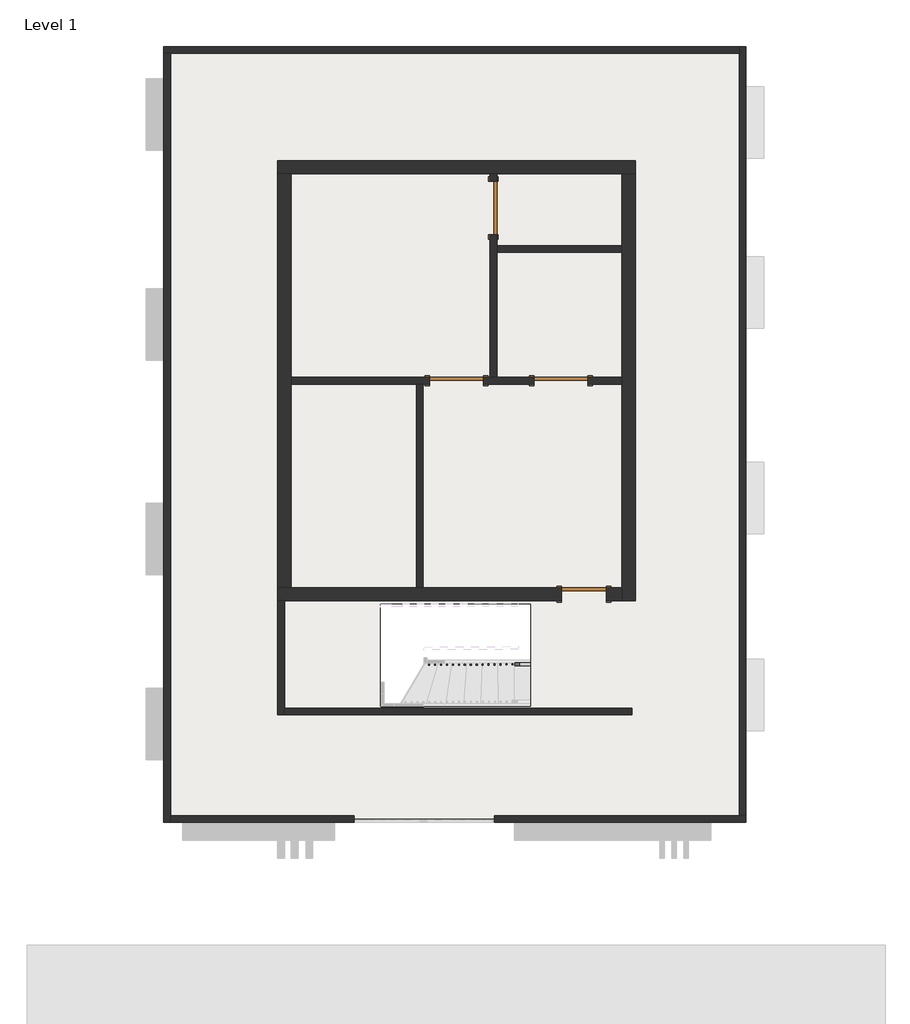
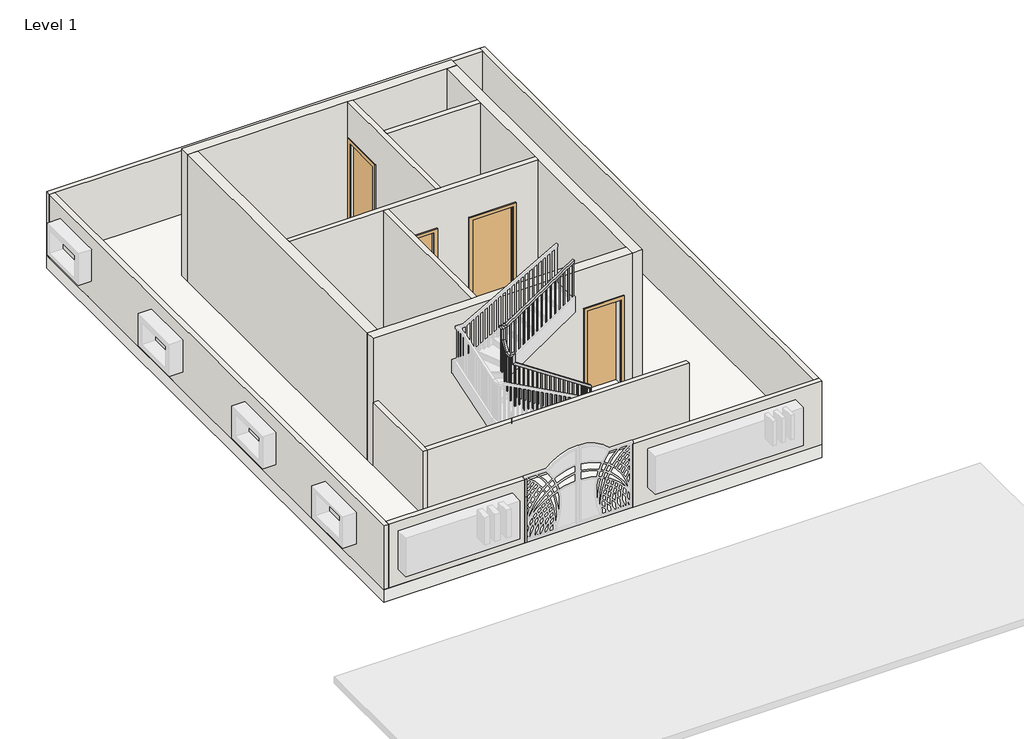
# One storey, part 1 of 2: 15 walls, 4 doors, 1 railing, 1 slab.
"""IFC4 building model written with IfcOpenShell, lengths in millimetres."""

from ifc_helpers import new_model, si_unit, frame, origin, origin_with_axes, place, context, project, spatial, polyline, outline, extrude, faceted_brep, transform, mapped, element, save
from components import door_a1484949, door_e5f9f3c4, door_305aa2a5

model = new_model("IFC4")

# Units and contexts
model_context = context("Model", 3, world=origin())
ifc_project = project(units=[si_unit("LENGTHUNIT", "METRE", prefix="MILLI")], contexts=[model_context])

# Site, building, storey
site = spatial("IfcSite", under=ifc_project)
building = spatial("IfcBuilding", under=site)
storey = spatial("IfcBuildingStorey", under=building, Name="Level 1", Elevation=0.0)

# Doors
placement = place(None, origin())
door_shape = door_a1484949(model_context)
element("IfcDoor", 1, ObjectType="Single-Flush : 30\" x 80\"", at=placement, inside=storey, context=model_context, shape_type="MappedRepresentation", body=[
    mapped(door_shape, transform((792.5410386, -2372.0109248, 0.0), x_axis=(1.0, 0.0, 0.0), y_axis=(0.0, 1.0, 0.0), z_axis=(0.0, 0.0, 1.0))),
])
door_2_shape = door_e5f9f3c4(model_context)
element("IfcDoor", 2, ObjectType="Single-Flush : 36\" x 84\"", at=placement, inside=storey, context=model_context, shape_type="MappedRepresentation", body=[
    mapped(door_2_shape, transform((-750.5089614, 4209.7640752, 0.0), x_axis=(0.0, -1.0, 0.0), y_axis=(1.0, 0.0, 0.0), z_axis=(0.0, 0.0, 1.0))),
])
door_3_shape = door_305aa2a5(model_context)
element("IfcDoor", 3, ObjectType="Single-Flush : 36\" x 84\"", at=placement, inside=storey, context=model_context, shape_type="MappedRepresentation", body=[
    mapped(door_3_shape, transform((402.0160386, 1266.5390752, 0.0), x_axis=(-1.0, 0.0, 0.0), y_axis=(0.0, -1.0, 0.0), z_axis=(0.0, 0.0, 1.0))),
])
element("IfcDoor", 4, ObjectType="Single-Flush : 36\" x 84\"", at=placement, inside=storey, context=model_context, shape_type="MappedRepresentation", body=[
    mapped(door_3_shape, transform((-1379.1589614, 1266.5390752, 0.0), x_axis=(-1.0, 0.0, 0.0), y_axis=(0.0, -1.0, 0.0), z_axis=(0.0, 0.0, 1.0))),
])

# Railing
element("IfcRailing", 5, ObjectType="Handrail - Rectangular", at=placement, inside=storey, context=model_context, shape_type="SolidModel", body=[
    faceted_brep([(-120.3816305, -3590.4209536, 1083.7333333), (-120.3816305, -3590.4209536, 1022.5630107), (-120.6930289, -3539.621908, 1022.5630107), (-120.6930289, -3539.621908, 1083.7333333), (-1854.5612186, -3601.0514854, 2247.0182998), (-1905.3602642, -3601.3628839, 2219.9238978), (-1905.6716627, -3550.5638383, 2219.9238978), (-1854.8726171, -3550.2524399, 2247.0182998), (-1854.5612186, -3601.0514854, 2469.2829276), (-1905.3602642, -3601.3628839, 2418.4829276), (-1905.6716627, -3550.5638383, 2418.4829276), (-1854.8726171, -3550.2524399, 2469.2829276), (-1981.5588325, -3601.8299816, 2469.2829276), (-1981.5588325, -3601.8299816, 2418.4829276), (-1931.0711854, -3550.7195376, 2418.4829276), (-1931.0711854, -3550.7195376, 2469.2829276), (-1982.3373287, -3474.8323677, 2469.2829276), (-1982.5128182, -3446.2044317, 2418.4829276), (-1931.7137726, -3445.8930332, 2418.4829276), (-1931.5382832, -3474.5209692, 2469.2829276), (-1983.1158249, -3347.8347538, 2679.0434812), (-1983.4272234, -3297.0357082, 2664.8632575), (-1932.6281778, -3296.7243097, 2664.8632575), (-1932.3167793, -3347.5233553, 2679.0434812), (-1983.1158249, -3347.8347538, 2950.4951436), (-1983.4272234, -3297.0357082, 2899.6951436), (-1932.6281778, -3296.7243097, 2899.6951436), (-1932.3167793, -3347.5233553, 2950.4951436), (-1983.8943211, -3220.8371398, 2950.4951436), (-1983.8943211, -3220.8371398, 2899.6951436), (-1932.783877, -3271.3247869, 2899.6951436), (-1932.783877, -3271.3247869, 2950.4951436), (-1856.8967072, -3220.0586437, 2950.4951436), (-1841.6341703, -3219.9650842, 2899.6951436), (-1841.3227719, -3270.7641298, 2899.6951436), (-1856.5853087, -3270.8576892, 2950.4951436), (-324.9523945, -3210.6678153, 3962.4), (-324.6409961, -3261.4668609, 3962.4), (-324.6409961, -3261.4668609, 3901.5185401), (-324.9523945, -3210.6678153, 3901.5185401)], [[[0, 1, 2, 3]], [[1, 0, 4, 5]], [[2, 1, 5, 6]], [[3, 2, 6, 7]], [[0, 3, 7, 4]], [[5, 4, 8, 9]], [[6, 5, 9, 10]], [[7, 6, 10, 11]], [[4, 7, 11, 8]], [[9, 8, 12, 13]], [[10, 9, 13, 14]], [[11, 10, 14, 15]], [[8, 11, 15, 12]], [[13, 12, 16, 17]], [[14, 13, 17, 18]], [[15, 14, 18, 19]], [[12, 15, 19, 16]], [[17, 16, 20, 21]], [[18, 17, 21, 22]], [[19, 18, 22, 23]], [[16, 19, 23, 20]], [[21, 20, 24, 25]], [[22, 21, 25, 26]], [[23, 22, 26, 27]], [[20, 23, 27, 24]], [[25, 24, 28, 29]], [[26, 25, 29, 30]], [[27, 26, 30, 31]], [[24, 27, 31, 28]], [[29, 28, 32, 33]], [[30, 29, 33, 34]], [[31, 30, 34, 35]], [[28, 31, 35, 32]], [[36, 37, 38, 39]], [[33, 32, 36, 39]], [[34, 33, 39, 38]], [[35, 34, 38, 37]], [[32, 35, 37, 36]]]),
    extrude(outline(polyline([(222.3085098, -19.05), (234.8914903, 0.0), (1246.1854534, 0.0), (1246.1854534, -19.05), (222.3085098, -19.05)])), frame((-342.2360746, -3245.6994205, 4124.8521201), z_axis=(-0.00612989118043648, 0.9999812120405643, 0.0), x_axis=(0.0, 0.0, -1.0)), (0.0, 0.0, 1.0), 19.05),
    extrude(outline(polyline([(222.3085098, -19.0499999), (234.8914902, 0.0), (1179.0762243, 0.0), (1179.0762243, -19.0499999), (222.3085098, -19.0499999)])), frame((-443.8341657, -3246.3222175, 4057.742891), z_axis=(-0.00612989118043648, 0.9999812120405643, 0.0), x_axis=(0.0, 0.0, -1.0)), (0.0, 0.0, 1.0), 19.05),
    extrude(outline(polyline([(222.3085098, -19.05), (234.8914902, 0.0), (1111.9669952, 0.0), (1111.9669952, -19.05), (222.3085098, -19.05)])), frame((-545.4322569, -3246.9450144, 3990.6336619), z_axis=(-0.00612989118043648, 0.9999812120405643, 0.0), x_axis=(0.0, 0.0, -1.0)), (0.0, 0.0, 1.0), 19.05),
    extrude(outline(polyline([(222.3085098, -19.05), (234.8914902, 0.0), (1214.1910995, 0.0), (1214.1910995, -19.05), (222.3085098, -19.05)])), frame((-647.030348, -3247.5678114, 3923.5244328), z_axis=(-0.00612989118043648, 0.9999812120405643, 0.0), x_axis=(0.0, 0.0, -1.0)), (0.0, 0.0, 1.0), 19.05),
    extrude(outline(polyline([(222.3085098, -19.05), (234.8914902, 0.0), (1147.0818704, 0.0), (1147.0818704, -19.05), (222.3085098, -19.05)])), frame((-748.6284392, -3248.1906083, 3856.4152037), z_axis=(-0.00612989118043648, 0.9999812120405643, 0.0), x_axis=(0.0, 0.0, -1.0)), (0.0, 0.0, 1.0), 19.05),
    extrude(outline(polyline([(222.3085098, -19.05), (234.8914902, 0.0), (1079.9726413, 0.0), (1079.9726413, -19.05), (222.3085098, -19.05)])), frame((-850.2265303, -3248.8134053, 3789.3059746), z_axis=(-0.00612989118043648, 0.9999812120405643, 0.0), x_axis=(0.0, 0.0, -1.0)), (0.0, 0.0, 1.0), 19.05),
    extrude(outline(polyline([(222.3085098, -19.05), (234.8914902, 0.0), (1182.1967455, 0.0), (1182.1967455, -19.05), (222.3085098, -19.05)])), frame((-951.8246215, -3249.4362022, 3722.1967455), z_axis=(-0.00612989118043648, 0.9999812120405643, 0.0), x_axis=(0.0, 0.0, -1.0)), (0.0, 0.0, 1.0), 19.05),
    extrude(outline(polyline([(222.3085097, -19.05), (234.8914902, 0.0), (1115.0875164, 0.0), (1115.0875164, -19.05), (222.3085097, -19.05)])), frame((-1053.4227126, -3250.0589992, 3655.0875164), z_axis=(-0.00612989118043648, 0.9999812120405643, 0.0), x_axis=(0.0, 0.0, -1.0)), (0.0, 0.0, 1.0), 19.05),
    extrude(outline(polyline([(222.3085097, -19.0499999), (234.8914902, 0.0), (1047.9782873, 0.0), (1047.9782873, -19.0499999), (222.3085097, -19.0499999)])), frame((-1155.0208037, -3250.6817961, 3587.9782873), z_axis=(-0.00612989118043648, 0.9999812120405643, 0.0), x_axis=(0.0, 0.0, -1.0)), (0.0, 0.0, 1.0), 19.05),
    extrude(outline(polyline([(222.3085097, -19.05), (234.8914902, 0.0), (1150.2023915, 0.0), (1150.2023915, -19.05), (222.3085097, -19.05)])), frame((-1256.6188949, -3251.304593, 3520.8690582), z_axis=(-0.00612989118043648, 0.9999812120405643, 0.0), x_axis=(0.0, 0.0, -1.0)), (0.0, 0.0, 1.0), 19.05),
    extrude(outline(polyline([(222.3085098, -19.05), (234.8914903, 0.0), (1083.0931625, 0.0), (1083.0931625, -19.05), (222.3085098, -19.05)])), frame((-1358.216986, -3251.92739, 3453.7598292), z_axis=(-0.00612989118043648, 0.9999812120405643, 0.0), x_axis=(0.0, 0.0, -1.0)), (0.0, 0.0, 1.0), 19.05),
    extrude(outline(polyline([(222.3085098, -19.05), (234.8914903, 0.0), (1185.3172668, 0.0), (1185.3172668, -19.05), (222.3085098, -19.05)])), frame((-1459.8150772, -3252.5501869, 3386.6506001), z_axis=(-0.00612989118043648, 0.9999812120405643, 0.0), x_axis=(0.0, 0.0, -1.0)), (0.0, 0.0, 1.0), 19.05),
    extrude(outline(polyline([(222.3085098, -19.05), (234.8914903, 0.0), (1118.2080377, 0.0), (1118.2080377, -19.05), (222.3085098, -19.05)])), frame((-1561.4131683, -3253.1729839, 3319.541371), z_axis=(-0.00612989118043648, 0.9999812120405643, 0.0), x_axis=(0.0, 0.0, -1.0)), (0.0, 0.0, 1.0), 19.05),
    extrude(outline(polyline([(222.3085098, -19.05), (234.8914902, 0.0), (1051.0988086, 0.0), (1051.0988086, -19.05), (222.3085098, -19.05)])), frame((-1663.0112595, -3253.7957808, 3252.4321419), z_axis=(-0.00612989118043648, 0.9999812120405643, 0.0), x_axis=(0.0, 0.0, -1.0)), (0.0, 0.0, 1.0), 19.05),
    extrude(outline(polyline([(222.3085098, -19.05), (234.8914902, 0.0), (1153.3229128, 0.0), (1153.3229128, -19.05), (222.3085098, -19.05)])), frame((-1764.6093506, -3254.4185778, 3185.3229128), z_axis=(-0.00612989118043648, 0.9999812120405643, 0.0), x_axis=(0.0, 0.0, -1.0)), (0.0, 0.0, 1.0), 19.05),
    extrude(outline(polyline([(222.3085098, -19.05), (234.8914902, 0.0), (1086.2136837, 0.0), (1086.2136837, -19.05), (222.3085098, -19.05)])), frame((-1866.2074418, -3255.0413747, 3118.2136837), z_axis=(-0.00612989118043648, 0.9999812120405643, 0.0), x_axis=(0.0, 0.0, -1.0)), (0.0, 0.0, 1.0), 19.05),
    extrude(outline(polyline([(-1948.6001916, -3280.94692), (-1967.6498337, -3281.0636944), (-1967.7666081, -3262.0140523), (-1948.716966, -3261.8972779), (-1948.6001916, -3280.94692)])), frame((0.0, 0.0, 1862.6666667), z_axis=(0.0, 0.0, 1.0), x_axis=(1.0, 0.0, 0.0)), (0.0, 0.0, 1.0), 1037.0284769),
    extrude(outline(polyline([(244.3320415, -19.05), (212.8679585, 0.0), (1074.2735921, 0.0), (1074.2735921, -19.05), (244.3320415, -19.05)])), frame((-1967.1438111, -3363.6121435, 2767.6069254), z_axis=(0.9999812120405644, 0.006129891180436036, 0.0), x_axis=(0.0, 0.0, -1.0)), (0.0, 0.0, 1.0), 19.05),
    extrude(outline(polyline([(244.3320415, -19.05), (212.8679585, 0.0), (1075.7984825, 0.0), (1075.7984825, -19.05), (244.3320415, -19.05)])), frame((-1966.5210142, -3465.2102346, 2599.7984825), z_axis=(0.9999812120405644, 0.006129891180436036, 0.0), x_axis=(0.0, 0.0, -1.0)), (0.0, 0.0, 1.0), 19.05),
    extrude(outline(polyline([(-1939.8365364, -3566.6485675), (-1939.719762, -3585.6982096), (-1958.7694041, -3585.814984), (-1958.8861785, -3566.7653419), (-1939.8365364, -3566.6485675)])), frame((0.0, 0.0, 1354.6666667), z_axis=(0.0, 0.0, 1.0), x_axis=(1.0, 0.0, 0.0)), (0.0, 0.0, 1.0), 1063.816261),
    extrude(outline(polyline([(234.9892351, -19.05), (222.2107648, 0.0), (1224.4109792, 0.0), (1224.4109792, -19.05), (234.9892351, -19.05)])), frame((-1857.171313, -3585.1921871, 2409.7443125), z_axis=(-0.006129891180436334, 0.9999812120405643, 0.0), x_axis=(0.0, 0.0, -1.0)), (0.0, 0.0, 1.0), 19.05),
    extrude(outline(polyline([(234.9892352, -19.05), (222.2107649, 0.0), (1156.259138, 0.0), (1156.259138, -19.05), (234.9892352, -19.05)])), frame((-1755.5732218, -3584.5693901, 2341.5924713), z_axis=(-0.006129891180436334, 0.9999812120405643, 0.0), x_axis=(0.0, 0.0, -1.0)), (0.0, 0.0, 1.0), 19.05),
    extrude(outline(polyline([(234.9892351, -19.05), (222.2107649, 0.0), (1257.44063, 0.0), (1257.44063, -19.05), (234.9892351, -19.05)])), frame((-1653.9751307, -3583.9465932, 2273.44063), z_axis=(-0.006129891180436334, 0.9999812120405643, 0.0), x_axis=(0.0, 0.0, -1.0)), (0.0, 0.0, 1.0), 19.05),
    extrude(outline(polyline([(234.9892351, -19.05), (222.2107649, 0.0), (1189.2887887, 0.0), (1189.2887887, -19.05), (234.9892351, -19.05)])), frame((-1552.3770395, -3583.3237962, 2205.2887887), z_axis=(-0.006129891180436334, 0.9999812120405643, 0.0), x_axis=(0.0, 0.0, -1.0)), (0.0, 0.0, 1.0), 19.05),
    extrude(outline(polyline([(234.9892351, -19.05), (222.2107649, 0.0), (1290.4702807, 0.0), (1290.4702807, -19.05), (234.9892351, -19.05)])), frame((-1450.7789484, -3582.7009993, 2137.1369474), z_axis=(-0.006129891180436334, 0.9999812120405643, 0.0), x_axis=(0.0, 0.0, -1.0)), (0.0, 0.0, 1.0), 19.05),
    extrude(outline(polyline([(234.9892351, -19.0499999), (222.2107649, 0.0), (1222.3184394, 0.0), (1222.3184394, -19.0499999), (234.9892351, -19.0499999)])), frame((-1349.1808572, -3582.0782024, 2068.9851061), z_axis=(-0.006129891180436334, 0.9999812120405643, 0.0), x_axis=(0.0, 0.0, -1.0)), (0.0, 0.0, 1.0), 19.05),
    extrude(outline(polyline([(234.9892351, -19.05), (222.2107648, 0.0), (1154.1665981, 0.0), (1154.1665981, -19.05), (234.9892351, -19.05)])), frame((-1247.5827661, -3581.4554054, 2000.8332648), z_axis=(-0.006129891180436334, 0.9999812120405643, 0.0), x_axis=(0.0, 0.0, -1.0)), (0.0, 0.0, 1.0), 19.05),
    extrude(outline(polyline([(234.9892352, -19.05), (222.2107649, 0.0), (1255.3480903, 0.0), (1255.3480903, -19.05), (234.9892352, -19.05)])), frame((-1145.984675, -3580.8326085, 1932.6814236), z_axis=(-0.006129891180436334, 0.9999812120405643, 0.0), x_axis=(0.0, 0.0, -1.0)), (0.0, 0.0, 1.0), 19.05),
    extrude(outline(polyline([(234.9892351, -19.05), (222.2107649, 0.0), (1187.196249, 0.0), (1187.196249, -19.05), (234.9892351, -19.05)])), frame((-1044.3865838, -3580.2098115, 1864.5295823), z_axis=(-0.006129891180436334, 0.9999812120405643, 0.0), x_axis=(0.0, 0.0, -1.0)), (0.0, 0.0, 1.0), 19.05),
    extrude(outline(polyline([(234.9892351, -19.05), (222.2107649, 0.0), (1288.377741, 0.0), (1288.377741, -19.05), (234.9892351, -19.05)])), frame((-942.7884927, -3579.5870146, 1796.377741), z_axis=(-0.006129891180436334, 0.9999812120405643, 0.0), x_axis=(0.0, 0.0, -1.0)), (0.0, 0.0, 1.0), 19.05),
    extrude(outline(polyline([(234.9892351, -19.05), (222.2107649, 0.0), (1220.2258997, 0.0), (1220.2258997, -19.05), (234.9892351, -19.05)])), frame((-841.1904015, -3578.9642176, 1728.2258997), z_axis=(-0.006129891180436334, 0.9999812120405643, 0.0), x_axis=(0.0, 0.0, -1.0)), (0.0, 0.0, 1.0), 19.05),
    extrude(outline(polyline([(234.9892351, -19.05), (222.2107649, 0.0), (1152.0740584, 0.0), (1152.0740584, -19.05), (234.9892351, -19.05)])), frame((-739.5923104, -3578.3414207, 1660.0740584), z_axis=(-0.006129891180436334, 0.9999812120405643, 0.0), x_axis=(0.0, 0.0, -1.0)), (0.0, 0.0, 1.0), 19.05),
    extrude(outline(polyline([(234.9892351, -19.0499999), (222.2107648, 0.0), (1253.2555504, 0.0), (1253.2555504, -19.0499999), (234.9892351, -19.0499999)])), frame((-637.9942192, -3577.7186237, 1591.9222171), z_axis=(-0.006129891180436334, 0.9999812120405643, 0.0), x_axis=(0.0, 0.0, -1.0)), (0.0, 0.0, 1.0), 19.05),
    extrude(outline(polyline([(234.9892352, -19.05), (222.2107649, 0.0), (1185.1037092, 0.0), (1185.1037092, -19.05), (234.9892352, -19.05)])), frame((-536.3961281, -3577.0958268, 1523.7703759), z_axis=(-0.006129891180436334, 0.9999812120405643, 0.0), x_axis=(0.0, 0.0, -1.0)), (0.0, 0.0, 1.0), 19.05),
    extrude(outline(polyline([(234.9892351, -19.05), (222.2107649, 0.0), (1116.9518679, 0.0), (1116.9518679, -19.05), (234.9892351, -19.05)])), frame((-434.798037, -3576.4730299, 1455.6185346), z_axis=(-0.006129891180436334, 0.9999812120405643, 0.0), x_axis=(0.0, 0.0, -1.0)), (0.0, 0.0, 1.0), 19.05),
    extrude(outline(polyline([(234.9892351, -19.05), (222.2107649, 0.0), (1218.13336, 0.0), (1218.13336, -19.05), (234.9892351, -19.05)])), frame((-333.1999458, -3575.8502329, 1387.4666933), z_axis=(-0.006129891180436334, 0.9999812120405643, 0.0), x_axis=(0.0, 0.0, -1.0)), (0.0, 0.0, 1.0), 19.05),
    extrude(outline(polyline([(234.9892351, -19.05), (222.2107649, 0.0), (1149.9815187, 0.0), (1149.9815187, -19.05), (234.9892351, -19.05)])), frame((-231.6018547, -3575.227436, 1319.314852), z_axis=(-0.006129891180436334, 0.9999812120405643, 0.0), x_axis=(0.0, 0.0, -1.0)), (0.0, 0.0, 1.0), 19.05),
    extrude(outline(polyline([(-1948.7558908, -3255.5473972), (-1967.8055329, -3255.6641716), (-1967.9223073, -3236.6145296), (-1948.8726652, -3236.4977551), (-1948.7558908, -3255.5473972)])), frame((0.0, 0.0, 1862.6666667), z_axis=(0.0, 0.0, 1.0), x_axis=(1.0, 0.0, 0.0)), (0.0, 0.0, 1.0), 1037.0284769),
    extrude(outline(polyline([(-1946.8485752, -3566.6915513), (-1946.7318007, -3585.7411934), (-1965.7814428, -3585.8579679), (-1965.8982173, -3566.8083258), (-1946.8485752, -3566.6915513)])), frame((0.0, 0.0, 1354.6666667), z_axis=(0.0, 0.0, 1.0), x_axis=(1.0, 0.0, 0.0)), (0.0, 0.0, 1.0), 1063.816261),
    extrude(outline(polyline([(222.3085098, -19.05), (234.8914902, 0.0), (1245.1603832, 0.0), (1245.1603832, -19.05), (222.3085098, -19.05)])), frame((-343.7879502, -3245.7089335, 4123.8270499), z_axis=(-0.00612989118043648, 0.9999812120405643, 0.0), x_axis=(0.0, 0.0, -1.0)), (0.0, 0.0, 1.0), 19.05),
    extrude(outline(polyline([(234.9892351, -19.05), (222.2107648, 0.0), (1088.2189125, 0.0), (1088.2189125, -19.05), (234.9892351, -19.05)])), frame((-139.5285846, -3574.6630262, 1257.5522458), z_axis=(-0.006129891180436334, 0.9999812120405643, 0.0), x_axis=(0.0, 0.0, -1.0)), (0.0, 0.0, 1.0), 19.05),
])

# Slab
element("IfcSlab", 6, ObjectType="Generic - 12\"", at=placement, inside=storey, context=model_context, shape_type="SweptSolid", body=[
    extrude(outline(polyline([(3554.7910386, 6962.4890752), (3554.7910386, -6258.2109248), (-6370.2589614, -6258.2109248), (-6370.2589614, 6962.4890752), (3554.7910386, 6962.4890752)]), holes=[polyline([(-116.1777511, -2539.253904), (-2673.8853157, -2539.253904), (-2673.8853157, -4276.2080688), (-116.1777511, -4276.2080688), (-116.1777511, -2539.253904)])]), frame((0.0, 0.0, -304.8), z_axis=(0.0, 0.0, 1.0), x_axis=(1.0, 0.0, 0.0)), (0.0, 0.0, 1.0), 304.8),
])

# Walls
element("IfcWall", 7, ObjectType="4.5\"", at=placement, inside=storey, context=model_context, shape_type="Brep", body=[
    faceted_brep([(-807.6589614, 3752.5640752, 2133.6), (-807.6589614, 3752.5640752, 0.0), (-807.6589614, 1323.6890752, 0.0), (-807.6589614, 1323.6890752, 3048.0), (-807.6589614, 4790.7890752, 3048.0), (-807.6589614, 4790.7890752, 0.0), (-807.6589614, 4666.9640752, 0.0), (-807.6589614, 4666.9640752, 2133.6), (-693.3589614, 1323.6890752, 0.0), (-693.3589614, 3457.2890752, 0.0), (-693.3589614, 3571.5890752, 0.0), (-693.3589614, 3752.5640752, 0.0), (-693.3589614, 3752.5640752, 2133.6), (-693.3589614, 4666.9640752, 2133.6), (-693.3589614, 4666.9640752, 0.0), (-693.3589614, 4790.7890752, 0.0), (-693.3589614, 4790.7890752, 3048.0), (-693.3589614, 3571.5890752, 3048.0), (-693.3589614, 3457.2890752, 3048.0), (-693.3589614, 1323.6890752, 3048.0)], [[[0, 1, 2, 3, 4, 5, 6, 7]], [[8, 9, 10, 11, 12, 13, 14, 15, 16, 17, 18, 19]], [[6, 5, 15, 14]], [[2, 1, 11, 10, 9, 8]], [[5, 4, 16, 15]], [[3, 2, 8, 19]], [[12, 11, 1, 0]], [[13, 12, 0, 7]], [[14, 13, 7, 6]], [[4, 3, 19, 18, 17, 16]]]),
])
element("IfcWall", 8, ObjectType="4.5\"", at=placement, inside=storey, context=model_context, shape_type="SweptSolid", body=[
    extrude(outline(polyline([(-693.3589614, 3571.5890752), (1440.2410386, 3571.5890752), (1440.2410386, 3457.2890752), (-693.3589614, 3457.2890752), (-693.3589614, 3571.5890752)])), origin_with_axes(), (0.0, 0.0, 1.0), 3048.0),
])
element("IfcWall", 9, ObjectType="4.5\"", at=placement, inside=storey, context=model_context, shape_type="Brep", body=[
    faceted_brep([(-4198.5589614, 1209.3890752, 0.0), (-2064.9589614, 1209.3890752, 0.0), (-1950.6589614, 1209.3890752, 0.0), (-1836.3589614, 1209.3890752, 0.0), (-1836.3589614, 1209.3890752, 2133.6), (-921.9589614, 1209.3890752, 2133.6), (-921.9589614, 1209.3890752, 0.0), (-55.1839614, 1209.3890752, 0.0), (-55.1839614, 1209.3890752, 2133.6), (859.2160386, 1209.3890752, 2133.6), (859.2160386, 1209.3890752, 0.0), (1440.2410386, 1209.3890752, 0.0), (1440.2410386, 1209.3890752, 3048.0), (-1950.6589614, 1209.3890752, 3048.0), (-2064.9589614, 1209.3890752, 3048.0), (-4198.5589614, 1209.3890752, 3048.0), (-1836.3589614, 1323.6890752, 2133.6), (-1836.3589614, 1323.6890752, 0.0), (-4198.5589614, 1323.6890752, 0.0), (-4198.5589614, 1323.6890752, 3048.0), (-807.6589614, 1323.6890752, 3048.0), (-693.3589614, 1323.6890752, 3048.0), (1440.2410386, 1323.6890752, 3048.0), (1440.2410386, 1323.6890752, 0.0), (859.2160386, 1323.6890752, 0.0), (859.2160386, 1323.6890752, 2133.6), (-55.1839614, 1323.6890752, 2133.6), (-55.1839614, 1323.6890752, 0.0), (-693.3589614, 1323.6890752, 0.0), (-807.6589614, 1323.6890752, 0.0), (-921.9589614, 1323.6890752, 0.0), (-921.9589614, 1323.6890752, 2133.6)], [[[0, 1, 2, 3, 4, 5, 6, 7, 8, 9, 10, 11, 12, 13, 14, 15]], [[16, 17, 18, 19, 20, 21, 22, 23, 24, 25, 26, 27, 28, 29, 30, 31]], [[24, 23, 11, 10]], [[18, 17, 3, 2, 1, 0]], [[30, 29, 28, 27, 7, 6]], [[12, 11, 23, 22]], [[0, 15, 19, 18]], [[8, 7, 27, 26]], [[9, 8, 26, 25]], [[10, 9, 25, 24]], [[4, 3, 17, 16]], [[5, 4, 16, 31]], [[6, 5, 31, 30]], [[15, 14, 13, 12, 22, 21, 20, 19]]]),
])
element("IfcWall", 10, ObjectType="4.5\"", at=placement, inside=storey, context=model_context, shape_type="SweptSolid", body=[
    extrude(outline(polyline([(-2064.9589614, -2257.7109248), (-2064.9589614, 1209.3890752), (-1950.6589614, 1209.3890752), (-1950.6589614, -2257.7109248), (-2064.9589614, -2257.7109248)])), origin_with_axes(), (0.0, 0.0, 1.0), 3048.0),
])
element("IfcWall", 11, ObjectType="4.5\"", at=placement, inside=storey, context=model_context, shape_type="Brep", body=[
    faceted_brep([(-4427.1589614, -2486.3109248, 0.0), (-4427.1589614, -4429.4109248, 0.0), (-4427.1589614, -4429.4109248, 1524.0), (-4427.1589614, -2486.3109248, 1524.0), (-4312.8589614, -2486.3109248, 0.0), (-4312.8589614, -2486.3109248, 1524.0), (-4312.8589614, -4315.1109248, 1524.0), (-4312.8589614, -4429.4109248, 1524.0), (-4312.8589614, -4429.4109248, 0.0), (-4312.8589614, -4315.1109248, 0.0)], [[[0, 1, 2, 3]], [[4, 5, 6, 7, 8, 9]], [[1, 0, 4, 9, 8]], [[3, 2, 7, 6, 5]], [[0, 3, 5, 4]], [[2, 1, 8, 7]]]),
])
element("IfcWall", 12, ObjectType="4.5\"", at=placement, inside=storey, context=model_context, shape_type="SweptSolid", body=[
    extrude(outline(polyline([(1611.6910386, -4429.4109248), (-4312.8589614, -4429.4109248), (-4312.8589614, -4315.1109248), (1611.6910386, -4315.1109248), (1611.6910386, -4429.4109248)])), origin_with_axes(), (0.0, 0.0, 1.0), 1524.0),
])
element("IfcWall", 13, ObjectType="4.5\"", at=placement, inside=storey, context=model_context, shape_type="Brep", body=[
    faceted_brep([(-6370.2589614, 6848.1890752, 0.0), (-6255.9589614, 6848.1890752, 0.0), (3440.4910386, 6848.1890752, 0.0), (3440.4910386, 6848.1890752, 1524.0), (-6255.9589614, 6848.1890752, 1524.0), (-6370.2589614, 6848.1890752, 1524.0), (-6370.2589614, 6962.4890752, 0.0), (-6370.2589614, 6962.4890752, 1524.0), (3440.4910386, 6962.4890752, 1524.0), (3440.4910386, 6962.4890752, 0.0)], [[[0, 1, 2, 3, 4, 5]], [[6, 7, 8, 9]], [[2, 1, 0, 6, 9]], [[5, 4, 3, 8, 7]], [[0, 5, 7, 6]], [[3, 2, 9, 8]]]),
])
element("IfcWall", 14, ObjectType="4.5\"", at=placement, inside=storey, context=model_context, shape_type="Brep", body=[
    faceted_brep([(-6255.9589614, -6258.2109248, 0.0), (-6255.9589614, -6143.9109248, 0.0), (-6255.9589614, 6848.1890752, 0.0), (-6255.9589614, 6848.1890752, 1524.0), (-6255.9589614, -6143.9109248, 1524.0), (-6255.9589614, -6258.2109248, 1524.0), (-6370.2589614, -6258.2109248, 0.0), (-6370.2589614, -6258.2109248, 1524.0), (-6370.2589614, 6848.1890752, 1524.0), (-6370.2589614, 6848.1890752, 0.0)], [[[0, 1, 2, 3, 4, 5]], [[6, 7, 8, 9]], [[2, 1, 0, 6, 9]], [[5, 4, 3, 8, 7]], [[0, 5, 7, 6]], [[3, 2, 9, 8]]]),
])
element("IfcWall", 15, ObjectType="4.5\"", at=placement, inside=storey, context=model_context, shape_type="Brep", body=[
    faceted_brep([(3554.7910386, -6143.9109248, 0.0), (3440.4910386, -6143.9109248, 0.0), (-731.4589614, -6143.9109248, 0.0), (-731.4589614, -6143.9109248, 1524.0), (3440.4910386, -6143.9109248, 1524.0), (3554.7910386, -6143.9109248, 1524.0), (3554.7910386, -6258.2109248, 0.0), (3554.7910386, -6258.2109248, 1524.0), (-731.4589614, -6258.2109248, 1524.0), (-731.4589614, -6258.2109248, 0.0)], [[[0, 1, 2, 3, 4, 5]], [[6, 7, 8, 9]], [[2, 1, 0, 6, 9]], [[3, 2, 9, 8]], [[5, 4, 3, 8, 7]], [[0, 5, 7, 6]]]),
])
element("IfcWall", 16, ObjectType="4.5\"", at=placement, inside=storey, context=model_context, shape_type="Brep", body=[
    faceted_brep([(3440.4910386, 6962.4890752, 0.0), (3440.4910386, 6848.1890752, 0.0), (3440.4910386, -6143.9109248, 0.0), (3440.4910386, -6143.9109248, 1524.0), (3440.4910386, 6848.1890752, 1524.0), (3440.4910386, 6962.4890752, 1524.0), (3554.7910386, 6962.4890752, 0.0), (3554.7910386, 6962.4890752, 1524.0), (3554.7910386, -6143.9109248, 1524.0), (3554.7910386, -6143.9109248, 0.0)], [[[0, 1, 2, 3, 4, 5]], [[6, 7, 8, 9]], [[2, 1, 0, 6, 9]], [[5, 4, 3, 8, 7]], [[0, 5, 7, 6]], [[3, 2, 9, 8]]]),
])
element("IfcWall", 17, ObjectType="4.5\"", at=placement, inside=storey, context=model_context, shape_type="SweptSolid", body=[
    extrude(outline(polyline([(-6255.9589614, -6143.9109248), (-3125.4089614, -6143.9109248), (-3125.4089614, -6258.2109248), (-6255.9589614, -6258.2109248), (-6255.9589614, -6143.9109248)])), origin_with_axes(), (0.0, 0.0, 1.0), 1524.0),
])
element("IfcWall", 18, ObjectType="9\"", at=placement, inside=storey, context=model_context, shape_type="Brep", body=[
    faceted_brep([(-4427.1589614, 4790.7890752, 0.0), (-4198.5589614, 4790.7890752, 0.0), (-807.6589614, 4790.7890752, 0.0), (-693.3589614, 4790.7890752, 0.0), (1440.2410386, 4790.7890752, 0.0), (1668.8410386, 4790.7890752, 0.0), (1668.8410386, 4790.7890752, 3048.0), (1440.2410386, 4790.7890752, 3048.0), (-693.3589614, 4790.7890752, 3048.0), (-807.6589614, 4790.7890752, 3048.0), (-4198.5589614, 4790.7890752, 3048.0), (-4427.1589614, 4790.7890752, 3048.0), (-4427.1589614, 5019.3890752, 0.0), (-4427.1589614, 5019.3890752, 3048.0), (1668.8410386, 5019.3890752, 3048.0), (1668.8410386, 5019.3890752, 0.0)], [[[0, 1, 2, 3, 4, 5, 6, 7, 8, 9, 10, 11]], [[12, 13, 14, 15]], [[5, 4, 3, 2, 1, 0, 12, 15]], [[6, 5, 15, 14]], [[0, 11, 13, 12]], [[11, 10, 9, 8, 7, 6, 14, 13]]]),
])
element("IfcWall", 19, ObjectType="9\"", at=placement, inside=storey, context=model_context, shape_type="Brep", body=[
    faceted_brep([(1440.2410386, 4790.7890752, 0.0), (1440.2410386, 3571.5890752, 0.0), (1440.2410386, 3457.2890752, 0.0), (1440.2410386, 1323.6890752, 0.0), (1440.2410386, 1209.3890752, 0.0), (1440.2410386, -2257.7109248, 0.0), (1440.2410386, -2486.3109248, 0.0), (1440.2410386, -2486.3109248, 3048.0), (1440.2410386, -2257.7109248, 3048.0), (1440.2410386, 1209.3890752, 3048.0), (1440.2410386, 1323.6890752, 3048.0), (1440.2410386, 3457.2890752, 3048.0), (1440.2410386, 3571.5890752, 3048.0), (1440.2410386, 4790.7890752, 3048.0), (1668.8410386, 4790.7890752, 0.0), (1668.8410386, 4790.7890752, 3048.0), (1668.8410386, -2486.3109248, 3048.0), (1668.8410386, -2486.3109248, 0.0)], [[[0, 1, 2, 3, 4, 5, 6, 7, 8, 9, 10, 11, 12, 13]], [[14, 15, 16, 17]], [[6, 5, 4, 3, 2, 1, 0, 14, 17]], [[0, 13, 15, 14]], [[7, 6, 17, 16]], [[13, 12, 11, 10, 9, 8, 7, 16, 15]]]),
])
element("IfcWall", 20, ObjectType="9\"", at=placement, inside=storey, context=model_context, shape_type="Brep", body=[
    faceted_brep([(1440.2410386, -2257.7109248, 0.0), (1173.5410386, -2257.7109248, 0.0), (1173.5410386, -2257.7109248, 2032.0), (411.5410386, -2257.7109248, 2032.0), (411.5410386, -2257.7109248, 0.0), (-1950.6589614, -2257.7109248, 0.0), (-2064.9589614, -2257.7109248, 0.0), (-4198.5589614, -2257.7109248, 0.0), (-4427.1589614, -2257.7109248, 0.0), (-4427.1589614, -2257.7109248, 3048.0), (-4198.5589614, -2257.7109248, 3048.0), (-2064.9589614, -2257.7109248, 3048.0), (-1950.6589614, -2257.7109248, 3048.0), (1440.2410386, -2257.7109248, 3048.0), (1173.5410386, -2486.3109248, 2032.0), (1173.5410386, -2486.3109248, 0.0), (1440.2410386, -2486.3109248, 0.0), (1440.2410386, -2486.3109248, 3048.0), (-4427.1589614, -2486.3109248, 3048.0), (-4427.1589614, -2486.3109248, 1524.0), (-4427.1589614, -2486.3109248, 0.0), (-4312.8589614, -2486.3109248, 0.0), (411.5410386, -2486.3109248, 0.0), (411.5410386, -2486.3109248, 2032.0)], [[[0, 1, 2, 3, 4, 5, 6, 7, 8, 9, 10, 11, 12, 13]], [[14, 15, 16, 17, 18, 19, 20, 21, 22, 23]], [[16, 15, 1, 0]], [[22, 21, 20, 8, 7, 6, 5, 4]], [[0, 13, 17, 16]], [[8, 20, 19, 18, 9]], [[2, 1, 15, 14]], [[3, 2, 14, 23]], [[4, 3, 23, 22]], [[13, 12, 11, 10, 9, 18, 17]]]),
])
element("IfcWall", 21, ObjectType="9\"", at=placement, inside=storey, context=model_context, shape_type="Brep", body=[
    faceted_brep([(-4198.5589614, -2257.7109248, 3048.0), (-4198.5589614, -2257.7109248, 0.0), (-4198.5589614, 1209.3890752, 0.0), (-4198.5589614, 1323.6890752, 0.0), (-4198.5589614, 4790.7890752, 0.0), (-4198.5589614, 4790.7890752, 3048.0), (-4198.5589614, 1323.6890752, 3048.0), (-4198.5589614, 1209.3890752, 3048.0), (-4427.1589614, -2257.7109248, 0.0), (-4427.1589614, -2257.7109248, 3048.0), (-4427.1589614, 4790.7890752, 3048.0), (-4427.1589614, 4790.7890752, 0.0)], [[[0, 1, 2, 3, 4, 5, 6, 7]], [[8, 9, 10, 11]], [[4, 3, 2, 1, 8, 11]], [[5, 4, 11, 10]], [[0, 9, 8, 1]], [[0, 7, 6, 5, 10, 9]]]),
])

save(model, "model.ifc")

# Revit data of these elements
# Type "Single-Flush : 30\" x 80\""
#   Type Mark = "5"
#   Construction Type Id = "MDOOR"
#   Assembly Code = "C1020"
#   Analytic Construction = "Metal"
#   Thickness = 0' - 2"
#   Heat Transfer Coefficient (U) = 0.651978 BTU/(h·ft²·°F)
#   Height = 6' - 8"
#   Trim Projection Ext = 0' - 1"
#   Trim Projection Int = 0' - 1"
#   Trim Width = 0' - 3"
#   Width = 2' - 6"
#   Define Thermal Properties by = 1
#   Define Thermal Properties by = 1
#   Door Material = Door - Panel
#   Frame Material = Door - Frame
#   Visual Light Transmittance = 0
#   Solar Heat Gain Coefficient = 0
#   Function = (empty or 0)
#   Wall Closure = (empty or 0)
# Type "Single-Flush : 36\" x 84\""
#   Type Mark = "1"
#   Construction Type Id = "MDOOR"
#   Assembly Code = "C1020"
#   Analytic Construction = "Metal"
#   Thickness = 0' - 2"
#   Heat Transfer Coefficient (U) = 0.651978 BTU/(h·ft²·°F)
#   Height = 7' - 0"
#   Trim Projection Ext = 0' - 1"
#   Trim Projection Int = 0' - 1"
#   Trim Width = 0' - 3"
#   Width = 3' - 0"
#   Define Thermal Properties by = 1
#   Define Thermal Properties by = 1
#   Door Material = Door - Panel
#   Frame Material = Door - Frame
#   Visual Light Transmittance = 0
#   Solar Heat Gain Coefficient = 0
#   Function = (empty or 0)
#   Wall Closure = (empty or 0)
# Type "Handrail - Rectangular"
#   Assembly Code = "C2010400"
#   built-in parameter 1008612 = 0.0416667 (stored number, unit not read)
#   built-in parameter 1008611 = 0.0416667 (stored number, unit not read)
#   built-in parameter 1008609 = 0.333333 (stored number, unit not read)
#   built-in parameter 1008604 = 0.166667 (stored number, unit not read)
#   built-in parameter 1008603 = 0.166667 (stored number, unit not read)
#   Railing Height = 3' - 0"
#   built-in parameter 1008630 = 2
#   built-in parameter 1008610 = 2
#   built-in parameter 1008618 = Baluster - Square : 3/4"
# Type "Generic - 12\""
#   Assembly Code = "B1010"
#   Function = 0
#   Layers, outside or top first: 1' - 0" no material (function 1)
# Type "4.5\""
#   Assembly Code = "B2010"
#   Layers, outside or top first: 0' - 4 1/2" no material (function 1)
# Type "9\""
#   Assembly Code = "B2010"
#   Layers, outside or top first: 0' - 9" no material (function 1)
# Element 1 (IfcDoor, "Single-Flush : 30\" x 80\"")
#   Phase Created = New Construction
#   Materials on its faces: "Door - Frame", "Door - Panel"
# Elements 2, 3, 4 (IfcDoor, "Single-Flush : 36\" x 84\"")
#   Phase Created = New Construction
#   Materials on its faces: "Door - Frame", "Door - Panel"
# Element 5 (IfcRailing, "Handrail - Rectangular")
#   Phase Created = New Construction
# Element 6 (IfcSlab, "Generic - 12\"")
#   Height Offset From Level = 0' - 0"
#   Phase Created = New Construction
#   Materials on its faces: "Default Floor"
# Elements 7, 8, 9, 10 (IfcWall, "4.5\"")
#   Top Offset = 0' - 0"
#   Base Offset = 0' - 0"
#   Unconnected Height = 10' - 0"
#   wall height = 10' - 0"
#   Phase Created = New Construction
#   Base Constraint = Level 1
#   Materials on its faces: "Default Wall"
# Elements 11, 12 (IfcWall, "4.5\"")
#   Top Offset = 0' - 0"
#   Base Offset = 0' - 0"
#   Unconnected Height = 5' - 0"
#   wall height = 5' - 0"
#   Phase Created = New Construction
#   Base Constraint = Level 1
#   Materials on its faces: "Default Wall", "Door - Frame"
# Elements 13, 14, 15, 16, 17 (IfcWall, "4.5\"")
#   Top Offset = 0' - 0"
#   Base Offset = 0' - 0"
#   Unconnected Height = 5' - 0"
#   wall height = 5' - 0"
#   Phase Created = New Construction
#   Base Constraint = Level 1
#   Materials on its faces: "Default Wall", "Door - Panel"
# Elements 18, 19, 20, 21 (IfcWall, "9\"")
#   Top Offset = 0' - 0"
#   Base Offset = 0' - 0"
#   Unconnected Height = 10' - 0"
#   wall height = 10' - 0"
#   Phase Created = New Construction
#   Base Constraint = Level 1
#   Materials on its faces: "Default Wall", "Door - Frame"
# Materials
#   "Door - Panel": class "Wood", colour RGB 210 159 95, transparency 0, Cost = 0
#   "Door - Frame": colour RGB 118 70 51, transparency 0, Cost = 0
#   "Default Floor": colour RGB 128 128 128, transparency 0, Cost = 0
#   "Default Wall": colour RGB 128 128 128, transparency 0, Cost = 0
